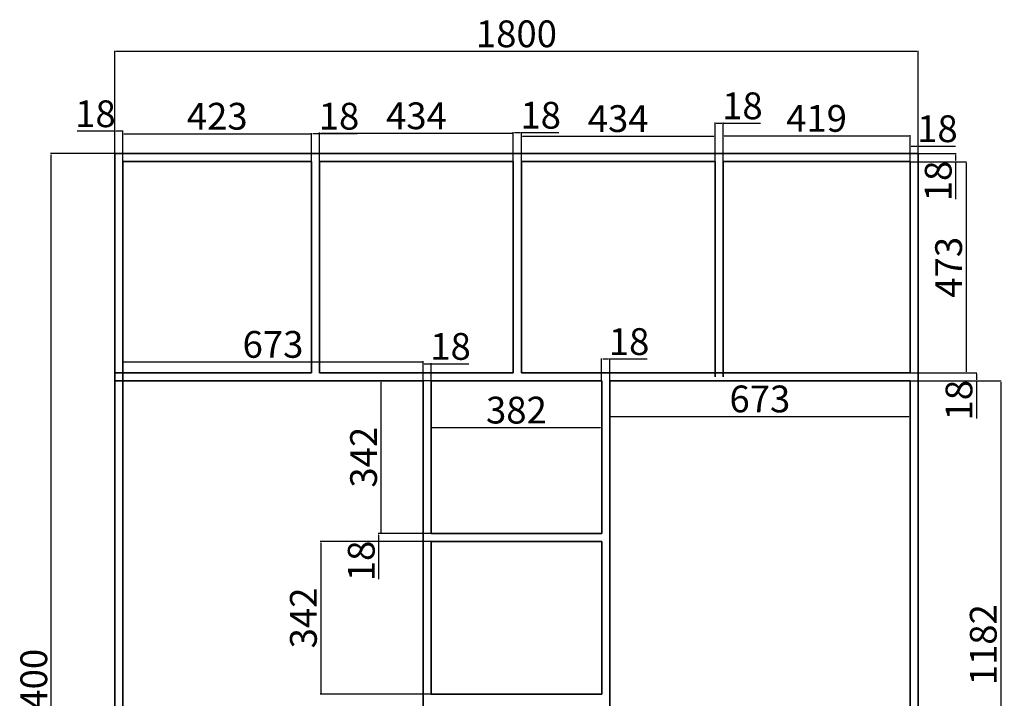
# Model space of a CAD drawing. Units: millimetres. Extents: x 222 to 5960, y 495 to 4622.
# Tile 2 of 3: x 616 to 2822, y 1826 to 3346. Entities that reach past the tile are written whole.
import ezdxf

# ---------------------------------------------------------------- set-up
doc = ezdxf.new("R2010")
doc.units = ezdxf.units.MM
doc.layers.add('A-ANNO-DIMS', color=2, linetype='Continuous', lineweight=18)
doc.layers.add('A-FURN', color=7, linetype='Continuous', lineweight=35)
doc.styles.get("Standard").update_dxf_attribs({"font": 'arial.ttf'})
doc.dimstyles.new('ISO-25', dxfattribs={"dimtxt": 60, "dimasz": 2.5, "dimexe": 1.25, "dimexo": 0.625, "dimtad": 1, "dimtxsty": 'Standard', "dimcen": 2.5, "dimadec": 0, "dimazin": 0, "dimtfac": 1, "dimtmove": 0, "dimatfit": 3, "dimfxl": 1, "dimarcsym": 0})

# ---------------------------------------------------------------- blocks, each defined once
blk = doc.blocks.new('*D1')
at = {"layer": 'A-ANNO-DIMS', "color": 0, "lineweight": -2, "transparency": 16777216}
for p, q in [((2610.8, 3028.3), (2610.8, 3063.7)), ((2613.3, 3062.4), (2626.3, 3062.4)), ((2628.8, 3028.3), (2628.8, 3063.7)), ((2628.8, 3062.4), (2713, 3062.4))]:
    blk.add_line(p, q, dxfattribs=at)
at = {"layer": 'A-ANNO-DIMS', "color": 0, "transparency": 16777216}
for points in [[(2613.3, 3062.8), (2613.3, 3062), (2610.8, 3062.4)], [(2626.3, 3062.8), (2626.3, 3062), (2628.8, 3062.4)]]:
    blk.add_solid(points, dxfattribs=at)
at = {"layer": 'Defpoints', "color": 0, "transparency": 16777216}
for p in [(2628.8, 3062.4), (2610.8, 3027.6), (2628.8, 3027.6)]:
    blk.add_point(p, dxfattribs=at)
at = {"layer": 'A-ANNO-DIMS', "color": 0, "transparency": 16777216, "insert": (2672.2, 3093.7), "char_height": 60, "attachment_point": 5}
blk.add_mtext('18', dxfattribs=at)
blk = doc.blocks.new('*D2')
at = {"layer": 'A-ANNO-DIMS', "color": 0, "lineweight": -2, "transparency": 16777216}
for p, q in [((2191.8, 3028.3), (2191.8, 3086.8)), ((2194.3, 3085.5), (2608.3, 3085.5)), ((2610.8, 3028.3), (2610.8, 3086.8))]:
    blk.add_line(p, q, dxfattribs=at)
at = {"layer": 'A-ANNO-DIMS', "color": 0, "transparency": 16777216}
for points in [[(2194.3, 3085.9), (2194.3, 3085.1), (2191.8, 3085.5)], [(2608.3, 3085.9), (2608.3, 3085.1), (2610.8, 3085.5)]]:
    blk.add_solid(points, dxfattribs=at)
at = {"layer": 'Defpoints', "color": 0, "transparency": 16777216}
for p in [(2610.8, 3085.5), (2191.8, 3027.6), (2610.8, 3027.6)]:
    blk.add_point(p, dxfattribs=at)
at = {"layer": 'A-ANNO-DIMS', "color": 0, "transparency": 16777216, "insert": (2401.3, 3116.8), "char_height": 60, "attachment_point": 5}
blk.add_mtext('419', dxfattribs=at)
blk = doc.blocks.new('*D3')
at = {"layer": 'A-ANNO-DIMS', "color": 0, "lineweight": -2, "transparency": 16777216}
for p, q in [((2173.8, 3028.3), (2173.8, 3115)), ((2176.3, 3113.8), (2189.3, 3113.8)), ((2191.8, 3028.3), (2191.8, 3115)), ((2191.8, 3113.8), (2276, 3113.8))]:
    blk.add_line(p, q, dxfattribs=at)
at = {"layer": 'A-ANNO-DIMS', "color": 0, "transparency": 16777216}
for points in [[(2176.3, 3114.2), (2176.3, 3113.3), (2173.8, 3113.8)], [(2189.3, 3114.2), (2189.3, 3113.3), (2191.8, 3113.8)]]:
    blk.add_solid(points, dxfattribs=at)
at = {"layer": 'Defpoints', "color": 0, "transparency": 16777216}
for p in [(2191.8, 3113.8), (2173.8, 3027.6), (2191.8, 3027.6)]:
    blk.add_point(p, dxfattribs=at)
at = {"layer": 'A-ANNO-DIMS', "color": 0, "transparency": 16777216, "insert": (2235.2, 3145), "char_height": 60, "attachment_point": 5}
blk.add_mtext('18', dxfattribs=at)
blk = doc.blocks.new('*D4')
at = {"layer": 'A-ANNO-DIMS', "color": 0, "lineweight": -2, "transparency": 16777216}
for p, q in [((1739.8, 3028.3), (1739.8, 3086.3)), ((1742.3, 3085), (2171.3, 3085)), ((2173.8, 3028.3), (2173.8, 3086.3))]:
    blk.add_line(p, q, dxfattribs=at)
at = {"layer": 'A-ANNO-DIMS', "color": 0, "transparency": 16777216}
for points in [[(1742.3, 3085.5), (1742.3, 3084.6), (1739.8, 3085)], [(2171.3, 3085.5), (2171.3, 3084.6), (2173.8, 3085)]]:
    blk.add_solid(points, dxfattribs=at)
at = {"layer": 'Defpoints', "color": 0, "transparency": 16777216}
for p in [(2173.8, 3085), (1739.8, 3027.6), (2173.8, 3027.6)]:
    blk.add_point(p, dxfattribs=at)
at = {"layer": 'A-ANNO-DIMS', "color": 0, "transparency": 16777216, "insert": (1956.8, 3116.3), "char_height": 60, "attachment_point": 5}
blk.add_mtext('434', dxfattribs=at)
blk = doc.blocks.new('*D5')
at = {"layer": 'A-ANNO-DIMS', "color": 0, "lineweight": -2, "transparency": 16777216}
for p, q in [((1721.8, 3028.3), (1721.8, 3093.9)), ((1724.3, 3092.7), (1737.3, 3092.7)), ((1739.8, 3028.3), (1739.8, 3093.9)), ((1739.8, 3092.7), (1824, 3092.7))]:
    blk.add_line(p, q, dxfattribs=at)
at = {"layer": 'A-ANNO-DIMS', "color": 0, "transparency": 16777216}
for points in [[(1724.3, 3093.1), (1724.3, 3092.3), (1721.8, 3092.7)], [(1737.3, 3093.1), (1737.3, 3092.3), (1739.8, 3092.7)]]:
    blk.add_solid(points, dxfattribs=at)
at = {"layer": 'Defpoints', "color": 0, "transparency": 16777216}
for p in [(1739.8, 3092.7), (1721.8, 3027.6), (1739.8, 3027.6)]:
    blk.add_point(p, dxfattribs=at)
at = {"layer": 'A-ANNO-DIMS', "color": 0, "transparency": 16777216, "insert": (1783.2, 3123.9), "char_height": 60, "attachment_point": 5}
blk.add_mtext('18', dxfattribs=at)
blk = doc.blocks.new('*D6')
at = {"layer": 'A-ANNO-DIMS', "color": 0, "lineweight": -2, "transparency": 16777216}
for p, q in [((1287.8, 3028.3), (1287.8, 3092.6)), ((1290.3, 3091.3), (1719.3, 3091.3)), ((1721.8, 3028.3), (1721.8, 3092.6))]:
    blk.add_line(p, q, dxfattribs=at)
at = {"layer": 'A-ANNO-DIMS', "color": 0, "transparency": 16777216}
for points in [[(1290.3, 3091.7), (1290.3, 3090.9), (1287.8, 3091.3)], [(1719.3, 3091.7), (1719.3, 3090.9), (1721.8, 3091.3)]]:
    blk.add_solid(points, dxfattribs=at)
at = {"layer": 'Defpoints', "color": 0, "transparency": 16777216}
for p in [(1721.8, 3091.3), (1287.8, 3027.6), (1721.8, 3027.6)]:
    blk.add_point(p, dxfattribs=at)
at = {"layer": 'A-ANNO-DIMS', "color": 0, "transparency": 16777216, "insert": (1504.8, 3122.6), "char_height": 60, "attachment_point": 5}
blk.add_mtext('434', dxfattribs=at)
blk = doc.blocks.new('*D7')
at = {"layer": 'A-ANNO-DIMS', "color": 0, "lineweight": -2, "transparency": 16777216}
for p, q in [((1269.8, 3028.3), (1269.8, 3091.7)), ((1272.3, 3090.5), (1285.3, 3090.5)), ((1287.8, 3028.3), (1287.8, 3091.7)), ((1287.8, 3090.5), (1372, 3090.5))]:
    blk.add_line(p, q, dxfattribs=at)
at = {"layer": 'A-ANNO-DIMS', "color": 0, "transparency": 16777216}
for points in [[(1272.3, 3090.9), (1272.3, 3090), (1269.8, 3090.5)], [(1285.3, 3090.9), (1285.3, 3090), (1287.8, 3090.5)]]:
    blk.add_solid(points, dxfattribs=at)
at = {"layer": 'Defpoints', "color": 0, "transparency": 16777216}
for p in [(1287.8, 3090.5), (1269.8, 3027.6), (1287.8, 3027.6)]:
    blk.add_point(p, dxfattribs=at)
at = {"layer": 'A-ANNO-DIMS', "color": 0, "transparency": 16777216, "insert": (1331.2, 3121.7), "char_height": 60, "attachment_point": 5}
blk.add_mtext('18', dxfattribs=at)
blk = doc.blocks.new('*D8')
at = {"layer": 'A-ANNO-DIMS', "color": 0, "lineweight": -2, "transparency": 16777216}
for p, q in [((846.8, 3028.3), (846.8, 3091.6)), ((849.3, 3090.3), (1267.3, 3090.3)), ((1269.8, 3028.3), (1269.8, 3091.6))]:
    blk.add_line(p, q, dxfattribs=at)
at = {"layer": 'A-ANNO-DIMS', "color": 0, "transparency": 16777216}
for points in [[(849.3, 3090.7), (849.3, 3089.9), (846.8, 3090.3)], [(1267.3, 3090.7), (1267.3, 3089.9), (1269.8, 3090.3)]]:
    blk.add_solid(points, dxfattribs=at)
at = {"layer": 'Defpoints', "color": 0, "transparency": 16777216}
for p in [(1269.8, 3090.3), (846.8, 3027.6), (1269.8, 3027.6)]:
    blk.add_point(p, dxfattribs=at)
at = {"layer": 'A-ANNO-DIMS', "color": 0, "transparency": 16777216, "insert": (1058.3, 3121.6), "char_height": 60, "attachment_point": 5}
blk.add_mtext('423', dxfattribs=at)
blk = doc.blocks.new('*D9')
at = {"layer": 'A-ANNO-DIMS', "color": 0, "lineweight": -2, "transparency": 16777216}
for p, q in [((828.8, 3095.9), (744.7, 3095.9)), ((828.8, 3028.3), (828.8, 3097.1)), ((844.3, 3095.9), (831.3, 3095.9)), ((846.8, 3028.3), (846.8, 3097.1))]:
    blk.add_line(p, q, dxfattribs=at)
at = {"layer": 'A-ANNO-DIMS', "color": 0, "transparency": 16777216}
for points in [[(831.3, 3096.3), (831.3, 3095.5), (828.8, 3095.9)], [(844.3, 3096.3), (844.3, 3095.5), (846.8, 3095.9)]]:
    blk.add_solid(points, dxfattribs=at)
at = {"layer": 'Defpoints', "color": 0, "transparency": 16777216}
for p in [(828.8, 3095.9), (828.8, 3027.6), (846.8, 3027.6)]:
    blk.add_point(p, dxfattribs=at)
at = {"layer": 'A-ANNO-DIMS', "color": 0, "transparency": 16777216, "insert": (785.5, 3127.2), "char_height": 60, "attachment_point": 5}
blk.add_mtext('18', dxfattribs=at)
blk = doc.blocks.new('*D10')
at = {"layer": 'A-ANNO-DIMS', "color": 0, "lineweight": -2, "transparency": 16777216}
for p, q in [((828.8, 3046.3), (828.8, 3276.2)), ((831.3, 3275), (2626.3, 3275)), ((2628.8, 3046.3), (2628.8, 3276.2))]:
    blk.add_line(p, q, dxfattribs=at)
at = {"layer": 'A-ANNO-DIMS', "color": 0, "transparency": 16777216}
for points in [[(831.3, 3275.4), (831.3, 3274.6), (828.8, 3275)], [(2626.3, 3275.4), (2626.3, 3274.6), (2628.8, 3275)]]:
    blk.add_solid(points, dxfattribs=at)
at = {"layer": 'Defpoints', "color": 0, "transparency": 16777216}
for p in [(2628.8, 3275), (828.8, 3045.6), (2628.8, 3045.6)]:
    blk.add_point(p, dxfattribs=at)
at = {"layer": 'A-ANNO-DIMS', "color": 0, "transparency": 16777216, "insert": (1728.8, 3306.2), "char_height": 60, "attachment_point": 5}
blk.add_mtext('1800', dxfattribs=at)
blk = doc.blocks.new('*D11')
at = {"layer": 'A-ANNO-DIMS', "color": 0, "lineweight": -2, "transparency": 16777216}
for p, q in [((2611.5, 3045.6), (2714.2, 3045.6)), ((2611.5, 3027.6), (2714.2, 3027.6)), ((2712.9, 3043.1), (2712.9, 3030.1)), ((2712.9, 3027.6), (2712.9, 2943.5))]:
    blk.add_line(p, q, dxfattribs=at)
at = {"layer": 'A-ANNO-DIMS', "color": 0, "transparency": 16777216}
for points in [[(2712.5, 3043.1), (2713.4, 3043.1), (2712.9, 3045.6)], [(2712.5, 3030.1), (2713.4, 3030.1), (2712.9, 3027.6)]]:
    blk.add_solid(points, dxfattribs=at)
at = {"layer": 'Defpoints', "color": 0, "transparency": 16777216}
for p in [(2610.8, 3045.6), (2610.8, 3027.6), (2712.9, 3027.6)]:
    blk.add_point(p, dxfattribs=at)
at = {"layer": 'A-ANNO-DIMS', "color": 0, "transparency": 16777216, "insert": (2681.7, 2984.3), "char_height": 60, "attachment_point": 5, "rotation": 90}
blk.add_mtext('18', dxfattribs=at)
blk = doc.blocks.new('*D12')
at = {"layer": 'A-ANNO-DIMS', "color": 0, "lineweight": -2, "transparency": 16777216}
for p, q in [((2611.5, 3027.6), (2737.5, 3027.6)), ((2736.3, 3025.1), (2736.3, 2557.1)), ((2611.5, 2554.6), (2737.5, 2554.6))]:
    blk.add_line(p, q, dxfattribs=at)
at = {"layer": 'A-ANNO-DIMS', "color": 0, "transparency": 16777216}
for points in [[(2735.9, 3025.1), (2736.7, 3025.1), (2736.3, 3027.6)], [(2735.9, 2557.1), (2736.7, 2557.1), (2736.3, 2554.6)]]:
    blk.add_solid(points, dxfattribs=at)
at = {"layer": 'Defpoints', "color": 0, "transparency": 16777216}
for p in [(2610.8, 3027.6), (2610.8, 2554.6), (2736.3, 2554.6)]:
    blk.add_point(p, dxfattribs=at)
at = {"layer": 'A-ANNO-DIMS', "color": 0, "transparency": 16777216, "insert": (2705, 2791.1), "char_height": 60, "attachment_point": 5, "rotation": 90}
blk.add_mtext('473', dxfattribs=at)
blk = doc.blocks.new('*D13')
at = {"layer": 'A-ANNO-DIMS', "color": 0, "lineweight": -2, "transparency": 16777216}
for p, q in [((2611.5, 2554.6), (2760.7, 2554.6)), ((2759.4, 2552.1), (2759.4, 2539.1)), ((2611.5, 2536.6), (2760.7, 2536.6)), ((2759.4, 2536.6), (2759.4, 2452.5))]:
    blk.add_line(p, q, dxfattribs=at)
at = {"layer": 'A-ANNO-DIMS', "color": 0, "transparency": 16777216}
for points in [[(2759, 2552.1), (2759.8, 2552.1), (2759.4, 2554.6)], [(2759, 2539.1), (2759.8, 2539.1), (2759.4, 2536.6)]]:
    blk.add_solid(points, dxfattribs=at)
at = {"layer": 'Defpoints', "color": 0, "transparency": 16777216}
for p in [(2610.8, 2554.6), (2610.8, 2536.6), (2759.4, 2536.6)]:
    blk.add_point(p, dxfattribs=at)
at = {"layer": 'A-ANNO-DIMS', "color": 0, "transparency": 16777216, "insert": (2728.2, 2493.3), "char_height": 60, "attachment_point": 5, "rotation": 90}
blk.add_mtext('18', dxfattribs=at)
blk = doc.blocks.new('*D14')
at = {"layer": 'A-ANNO-DIMS', "color": 0, "lineweight": -2, "transparency": 16777216}
for p, q in [((2611.5, 2536.6), (2815.2, 2536.6)), ((2813.9, 2534.1), (2813.9, 1357.1)), ((2611.5, 1354.6), (2815.2, 1354.6))]:
    blk.add_line(p, q, dxfattribs=at)
at = {"layer": 'A-ANNO-DIMS', "color": 0, "transparency": 16777216}
for points in [[(2813.5, 2534.1), (2814.3, 2534.1), (2813.9, 2536.6)], [(2813.5, 1357.1), (2814.3, 1357.1), (2813.9, 1354.6)]]:
    blk.add_solid(points, dxfattribs=at)
at = {"layer": 'Defpoints', "color": 0, "transparency": 16777216}
for p in [(2610.8, 2536.6), (2610.8, 1354.6), (2813.9, 1354.6)]:
    blk.add_point(p, dxfattribs=at)
at = {"layer": 'A-ANNO-DIMS', "color": 0, "transparency": 16777216, "insert": (2782.7, 1945.6), "char_height": 60, "attachment_point": 5, "rotation": 90}
blk.add_mtext('1182', dxfattribs=at)
blk = doc.blocks.new('*D16')
at = {"layer": 'A-ANNO-DIMS', "color": 0, "lineweight": -2, "transparency": 16777216}
for p, q in [((846.8, 2537.3), (846.8, 2580.5)), ((849.3, 2579.3), (1517.3, 2579.3)), ((1519.8, 2537.3), (1519.8, 2580.5))]:
    blk.add_line(p, q, dxfattribs=at)
at = {"layer": 'A-ANNO-DIMS', "color": 0, "transparency": 16777216}
for points in [[(849.3, 2579.7), (849.3, 2578.9), (846.8, 2579.3)], [(1517.3, 2579.7), (1517.3, 2578.9), (1519.8, 2579.3)]]:
    blk.add_solid(points, dxfattribs=at)
at = {"layer": 'Defpoints', "color": 0, "transparency": 16777216}
for p in [(1519.8, 2579.3), (846.8, 2536.6), (1519.8, 2536.6)]:
    blk.add_point(p, dxfattribs=at)
at = {"layer": 'A-ANNO-DIMS', "color": 0, "transparency": 16777216, "insert": (1183.3, 2610.6), "char_height": 60, "attachment_point": 5}
blk.add_mtext('673', dxfattribs=at)
blk = doc.blocks.new('*D17')
at = {"layer": 'A-ANNO-DIMS', "color": 0, "lineweight": -2, "transparency": 16777216}
for p, q in [((1519.8, 2537.3), (1519.8, 2576.1)), ((1522.3, 2574.8), (1535.3, 2574.8)), ((1537.8, 2537.3), (1537.8, 2576.1)), ((1537.8, 2574.8), (1622, 2574.8))]:
    blk.add_line(p, q, dxfattribs=at)
at = {"layer": 'A-ANNO-DIMS', "color": 0, "transparency": 16777216}
for points in [[(1522.3, 2575.2), (1522.3, 2574.4), (1519.8, 2574.8)], [(1535.3, 2575.2), (1535.3, 2574.4), (1537.8, 2574.8)]]:
    blk.add_solid(points, dxfattribs=at)
at = {"layer": 'Defpoints', "color": 0, "transparency": 16777216}
for p in [(1537.8, 2574.8), (1519.8, 2536.6), (1537.8, 2536.6)]:
    blk.add_point(p, dxfattribs=at)
at = {"layer": 'A-ANNO-DIMS', "color": 0, "transparency": 16777216, "insert": (1581.2, 2606.1), "char_height": 60, "attachment_point": 5}
blk.add_mtext('18', dxfattribs=at)
blk = doc.blocks.new('*D18')
at = {"layer": 'A-ANNO-DIMS', "color": 0, "lineweight": -2, "transparency": 16777216}
for p, q in [((1537.8, 2536), (1537.8, 2430.8)), ((1919.8, 2536), (1919.8, 2430.8)), ((1540.3, 2432.1), (1917.3, 2432.1))]:
    blk.add_line(p, q, dxfattribs=at)
at = {"layer": 'A-ANNO-DIMS', "color": 0, "transparency": 16777216}
for points in [[(1540.3, 2432.5), (1540.3, 2431.7), (1537.8, 2432.1)], [(1917.3, 2432.5), (1917.3, 2431.7), (1919.8, 2432.1)]]:
    blk.add_solid(points, dxfattribs=at)
at = {"layer": 'Defpoints', "color": 0, "transparency": 16777216}
for p in [(1537.8, 2536.6), (1919.8, 2536.6), (1919.8, 2432.1)]:
    blk.add_point(p, dxfattribs=at)
at = {"layer": 'A-ANNO-DIMS', "color": 0, "transparency": 16777216, "insert": (1728.8, 2463.4), "char_height": 60, "attachment_point": 5}
blk.add_mtext('382', dxfattribs=at)
blk = doc.blocks.new('*D19')
at = {"layer": 'A-ANNO-DIMS', "color": 0, "lineweight": -2, "transparency": 16777216}
for p, q in [((1919.8, 2537.3), (1919.8, 2586.9)), ((1922.3, 2585.7), (1935.3, 2585.7)), ((1937.8, 2537.3), (1937.8, 2586.9)), ((1937.8, 2585.7), (2022, 2585.7))]:
    blk.add_line(p, q, dxfattribs=at)
at = {"layer": 'A-ANNO-DIMS', "color": 0, "transparency": 16777216}
for points in [[(1922.3, 2586.1), (1922.3, 2585.2), (1919.8, 2585.7)], [(1935.3, 2586.1), (1935.3, 2585.2), (1937.8, 2585.7)]]:
    blk.add_solid(points, dxfattribs=at)
at = {"layer": 'Defpoints', "color": 0, "transparency": 16777216}
for p in [(1937.8, 2585.7), (1919.8, 2536.6), (1937.8, 2536.6)]:
    blk.add_point(p, dxfattribs=at)
at = {"layer": 'A-ANNO-DIMS', "color": 0, "transparency": 16777216, "insert": (1981.2, 2616.9), "char_height": 60, "attachment_point": 5}
blk.add_mtext('18', dxfattribs=at)
blk = doc.blocks.new('*D20')
at = {"layer": 'A-ANNO-DIMS', "color": 0, "lineweight": -2, "transparency": 16777216}
for p, q in [((1937.8, 2536), (1937.8, 2455.9)), ((2610.8, 2536), (2610.8, 2455.9)), ((1940.3, 2457.2), (2608.3, 2457.2))]:
    blk.add_line(p, q, dxfattribs=at)
at = {"layer": 'A-ANNO-DIMS', "color": 0, "transparency": 16777216}
for points in [[(1940.3, 2457.6), (1940.3, 2456.7), (1937.8, 2457.2)], [(2608.3, 2457.6), (2608.3, 2456.7), (2610.8, 2457.2)]]:
    blk.add_solid(points, dxfattribs=at)
at = {"layer": 'Defpoints', "color": 0, "transparency": 16777216}
for p in [(1937.8, 2536.6), (2610.8, 2536.6), (2610.8, 2457.2)]:
    blk.add_point(p, dxfattribs=at)
at = {"layer": 'A-ANNO-DIMS', "color": 0, "transparency": 16777216, "insert": (2274.3, 2488.4), "char_height": 60, "attachment_point": 5}
blk.add_mtext('673', dxfattribs=at)
blk = doc.blocks.new('*D21')
at = {"layer": 'A-ANNO-DIMS', "color": 0, "lineweight": -2, "transparency": 16777216}
for p, q in [((1537.2, 2536.6), (1424.2, 2536.6)), ((1425.4, 2197.1), (1425.4, 2534.1)), ((1537.2, 2194.6), (1424.2, 2194.6))]:
    blk.add_line(p, q, dxfattribs=at)
at = {"layer": 'A-ANNO-DIMS', "color": 0, "transparency": 16777216}
for points in [[(1425, 2534.1), (1425.8, 2534.1), (1425.4, 2536.6)], [(1425, 2197.1), (1425.8, 2197.1), (1425.4, 2194.6)]]:
    blk.add_solid(points, dxfattribs=at)
at = {"layer": 'Defpoints', "color": 0, "transparency": 16777216}
for p in [(1425.4, 2536.6), (1537.8, 2536.6), (1537.8, 2194.6)]:
    blk.add_point(p, dxfattribs=at)
at = {"layer": 'A-ANNO-DIMS', "color": 0, "transparency": 16777216, "insert": (1394.1, 2365.6), "char_height": 60, "attachment_point": 5, "rotation": 90}
blk.add_mtext('342', dxfattribs=at)
blk = doc.blocks.new('*D22')
at = {"layer": 'A-ANNO-DIMS', "color": 0, "lineweight": -2, "transparency": 16777216}
for p, q in [((1537.2, 2194.6), (1418.8, 2194.6)), ((1420, 2192.1), (1420, 2179.1)), ((1537.2, 2176.6), (1418.8, 2176.6)), ((1420, 2176.6), (1420, 2092.5))]:
    blk.add_line(p, q, dxfattribs=at)
at = {"layer": 'A-ANNO-DIMS', "color": 0, "transparency": 16777216}
for points in [[(1419.6, 2192.1), (1420.4, 2192.1), (1420, 2194.6)], [(1419.6, 2179.1), (1420.4, 2179.1), (1420, 2176.6)]]:
    blk.add_solid(points, dxfattribs=at)
at = {"layer": 'Defpoints', "color": 0, "transparency": 16777216}
for p in [(1537.8, 2194.6), (1420, 2176.6), (1537.8, 2176.6)]:
    blk.add_point(p, dxfattribs=at)
at = {"layer": 'A-ANNO-DIMS', "color": 0, "transparency": 16777216, "insert": (1388.8, 2133.3), "char_height": 60, "attachment_point": 5, "rotation": 90}
blk.add_mtext('18', dxfattribs=at)
blk = doc.blocks.new('*D23')
at = {"layer": 'A-ANNO-DIMS', "color": 0, "lineweight": -2, "transparency": 16777216}
for p, q in [((1537.2, 2176.6), (1289.2, 2176.6)), ((1290.4, 2174.1), (1290.4, 1837.1)), ((1537.2, 1834.6), (1289.2, 1834.6))]:
    blk.add_line(p, q, dxfattribs=at)
at = {"layer": 'A-ANNO-DIMS', "color": 0, "transparency": 16777216}
for points in [[(1290, 2174.1), (1290.9, 2174.1), (1290.4, 2176.6)], [(1290, 1837.1), (1290.9, 1837.1), (1290.4, 1834.6)]]:
    blk.add_solid(points, dxfattribs=at)
at = {"layer": 'Defpoints', "color": 0, "transparency": 16777216}
for p in [(1537.8, 2176.6), (1290.4, 1834.6), (1537.8, 1834.6)]:
    blk.add_point(p, dxfattribs=at)
at = {"layer": 'A-ANNO-DIMS', "color": 0, "transparency": 16777216, "insert": (1259.2, 2005.6), "char_height": 60, "attachment_point": 5, "rotation": 90}
blk.add_mtext('342', dxfattribs=at)
blk = doc.blocks.new('SHELF-COMPARTMENT')
for p, q in [((0, 342), (0, 0)), ((0, 342), (382, 342)), ((382, 342), (382, 0)), ((0, 0), (382, 0))]:
    blk.add_line(p, q)
blk = doc.blocks.new('*D59')
at = {"layer": 'A-ANNO-DIMS', "color": 0, "lineweight": -2, "transparency": 16777216}
for p, q in [((828.2, 3045.6), (685.1, 3045.6)), ((686.3, 648.1), (686.3, 3043.1)), ((828.2, 645.6), (685.1, 645.6))]:
    blk.add_line(p, q, dxfattribs=at)
at = {"layer": 'A-ANNO-DIMS', "color": 0, "transparency": 16777216}
for points in [[(685.9, 3043.1), (686.8, 3043.1), (686.3, 3045.6)], [(685.9, 648.1), (686.8, 648.1), (686.3, 645.6)]]:
    blk.add_solid(points, dxfattribs=at)
at = {"layer": 'Defpoints', "color": 0, "transparency": 16777216}
for p in [(686.3, 3045.6), (828.8, 3045.6), (828.8, 645.6)]:
    blk.add_point(p, dxfattribs=at)
at = {"layer": 'A-ANNO-DIMS', "color": 0, "transparency": 16777216, "insert": (655.1, 1845.6), "char_height": 60, "attachment_point": 5, "rotation": 90}
blk.add_mtext('2400', dxfattribs=at)

msp = doc.modelspace()

# ---------------------------------------------------------------- linework, layer by layer
at = {"layer": 'A-FURN'}
for p, q in [((2628.845, 3045.641), (828.845, 3045.641)), ((828.845, 3045.641), (828.845, 645.641)), ((828.845, 3045.641), (828.845, 2545.641)), ((2628.845, 645.641), (2628.845, 3045.641)), ((846.845, 3027.641), (846.845, 2545.641)), ((1269.845, 3027.641), (846.845, 3027.641)), ((1269.845, 3027.641), (1269.845, 2554.641)), ((1287.845, 3027.641), (1287.845, 2554.641)), ((1721.845, 3027.641), (1287.845, 3027.641)), ((1721.845, 3027.641), (1721.845, 2554.641)), ((1739.845, 3027.641), (1739.845, 2554.641)), ((2173.845, 3027.641), (1739.845, 3027.641)), ((2173.845, 3027.641), (2173.845, 2545.641)), ((2610.845, 3027.641), (2191.845, 3027.641)), ((2191.845, 3027.641), (2191.845, 2545.641)), ((2610.845, 2554.641), (2610.845, 3027.641)), ((828.845, 2554.641), (1269.845, 2554.641)), ((828.845, 2545.641), (828.845, 645.641)), ((846.845, 2545.641), (846.845, 1354.641)), ((1287.845, 2554.641), (1721.845, 2554.641)), ((1739.845, 2554.641), (2610.845, 2554.641)), ((828.845, 2536.641), (1519.845, 2536.641)), ((1519.845, 2536.641), (1519.845, 1354.641)), ((1937.845, 2536.641), (1937.845, 1354.641)), ((1937.845, 2536.641), (2610.845, 2536.641)), ((2610.845, 1354.641), (2610.845, 2536.641))]:
    msp.add_line(p, q, dxfattribs=at)

# ---------------------------------------------------------------- block references
msp.add_blockref('SHELF-COMPARTMENT', (1537.845, 2194.641), dxfattribs=at)
at = {"layer": 'A-FURN', "rotation": 180}
msp.add_blockref('SHELF-COMPARTMENT', (1919.845, 2176.641), dxfattribs=at)

# ---------------------------------------------------------------- dimensions: what is measured, and where the dimension line sits
at = {"layer": 'A-ANNO-DIMS'}
for base, p1, p2, picture, middle in [((2628.845, 3274.983), (828.845, 3045.641), (2628.845, 3045.641), '*D10', (1728.845, 3306.242)), ((2191.845, 3113.754), (2173.845, 3027.641), (2191.845, 3027.641), '*D3', (2235.181, 3145.014)), ((828.845, 3095.899), (846.845, 3027.641), (828.845, 3027.641), '*D9', (785.508, 3127.159)), ((1269.845, 3090.332), (846.845, 3027.641), (1269.845, 3027.641), '*D8', (1058.345, 3121.612)), ((1287.845, 3090.467), (1269.845, 3027.641), (1287.845, 3027.641), '*D7', (1331.181, 3121.726)), ((1721.845, 3091.31), (1287.845, 3027.641), (1721.845, 3027.641), '*D6', (1504.845, 3122.59)), ((1739.845, 3092.672), (1721.845, 3027.641), (1739.845, 3027.641), '*D5', (1783.181, 3123.931)), ((2173.845, 3085.036), (1739.845, 3027.641), (2173.845, 3027.641), '*D4', (1956.845, 3116.316)), ((2610.845, 3085.504), (2191.845, 3027.641), (2610.845, 3027.641), '*D2', (2401.345, 3116.763)), ((2628.845, 3062.429), (2610.845, 3027.641), (2628.845, 3027.641), '*D1', (2672.181, 3093.688)), ((1519.845, 2579.289), (846.845, 2536.641), (1519.845, 2536.641), '*D16', (1183.345, 2610.568)), ((1937.845, 2585.664), (1919.845, 2536.641), (1937.845, 2536.641), '*D19', (1981.181, 2616.923)), ((1537.845, 2574.812), (1519.845, 2536.641), (1537.845, 2536.641), '*D17', (1581.181, 2606.072)), ((1919.845, 2432.095), (1537.845, 2536.641), (1919.845, 2536.641), '*D18', (1728.845, 2463.375)), ((2610.845, 2457.155), (1937.845, 2536.641), (2610.845, 2536.641), '*D20', (2274.345, 2488.435))]:
    dim = msp.add_linear_dim(base=base, p1=p1, p2=p2, dimstyle='ISO-25', override={"dimclrd": 0, "dimclre": 0, "dimclrt": 0}, dxfattribs=at)
    dim.commit()
    dim.dimension.update_dxf_attribs({"geometry": picture, "text_midpoint": middle})
for base, p1, p2, override, picture, middle in [((686.345, 3045.641), (828.845, 645.641), (828.845, 3045.641), {"dimdec": 0, "dimlfac": 1, "dimrnd": 0, "dimzin": 0, "dimdsep": 46, "dimlunit": 2}, '*D59', (655.085, 1845.641)), ((2712.946, 3027.641), (2610.845, 3045.641), (2610.845, 3027.641), {"dimclrd": 0, "dimclre": 0, "dimclrt": 0}, '*D11', (2681.686, 2984.305)), ((2736.276, 2554.641), (2610.845, 3027.641), (2610.845, 2554.641), {"dimclrd": 0, "dimclre": 0, "dimclrt": 0}, '*D12', (2704.996, 2791.141)), ((2759.414, 2536.641), (2610.845, 2554.641), (2610.845, 2536.641), {"dimclrd": 0, "dimclre": 0, "dimclrt": 0}, '*D13', (2728.155, 2493.305)), ((1425.416, 2536.641), (1537.845, 2194.641), (1537.845, 2536.641), {"dimclrd": 0, "dimclre": 0, "dimclrt": 0}, '*D21', (1394.136, 2365.641)), ((2813.931, 1354.641), (2610.845, 2536.641), (2610.845, 1354.641), {"dimclrd": 0, "dimclre": 0, "dimclrt": 0}, '*D14', (2782.672, 1945.641)), ((1420.023, 2176.641), (1537.845, 2194.641), (1537.845, 2176.641), {"dimclrd": 0, "dimclre": 0, "dimclrt": 0}, '*D22', (1388.764, 2133.305)), ((1290.443, 1834.641), (1537.845, 2176.641), (1537.845, 1834.641), {"dimclrd": 0, "dimclre": 0, "dimclrt": 0}, '*D23', (1259.163, 2005.641))]:
    dim = msp.add_linear_dim(base=base, p1=p1, p2=p2, angle=90, dimstyle='ISO-25', override=override, dxfattribs=at)
    dim.commit()
    dim.dimension.update_dxf_attribs({"geometry": picture, "text_midpoint": middle})

doc.saveas('drawing.dxf')
